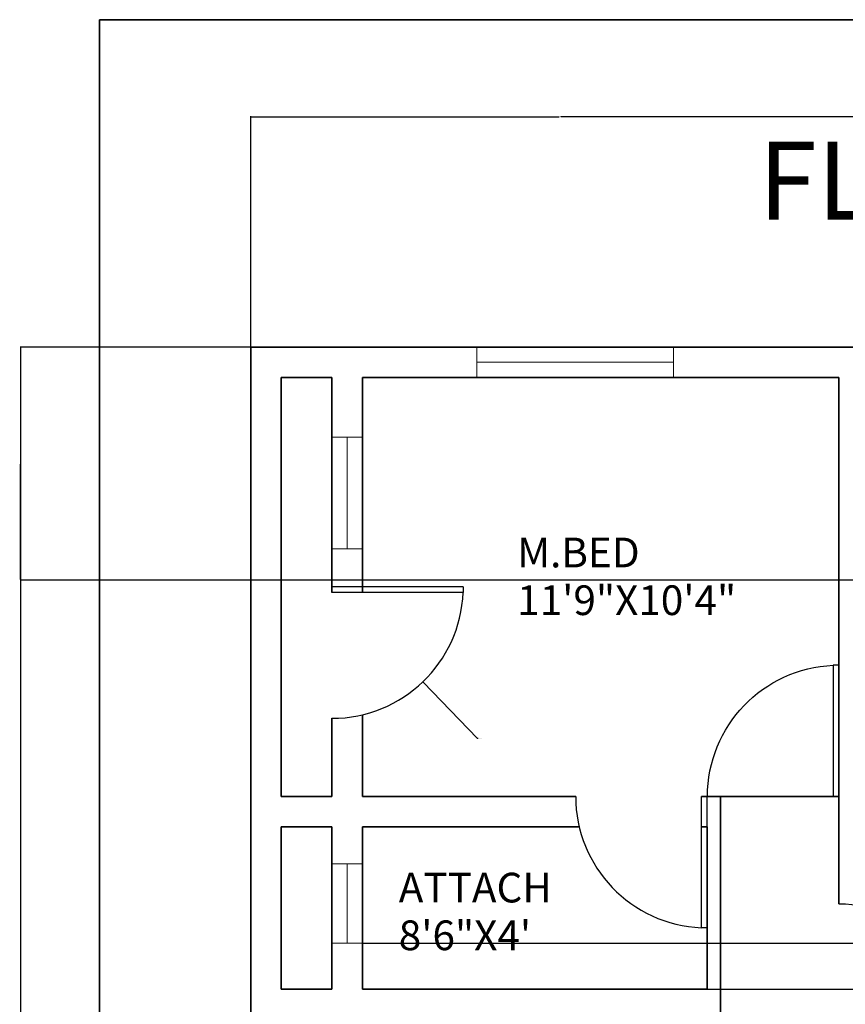
# Model space of a CAD drawing. Units: feet. Extents: x 100807 to 101423, y 154875 to 156331.
# Tile 3 of 8: x 100807 to 101051, y 156040 to 156331. Entities that reach past the tile are written whole.
import ezdxf

# ---------------------------------------------------------------- set-up
doc = ezdxf.new("R2010")
doc.units = ezdxf.units.FT
for name, color, linetype, lineweight in [('A-ANNO-DIMS', 2, 'Continuous', 18), ('A-ANNO-TITL', 7, 'Continuous', 35), ('A-ANNO-TTLB', 7, 'Continuous', 35), ('A-AREA-IDEN', 7, 'Continuous', 25), ('A-DOOR', 4, 'Continuous', 25), ('A-GLAZ', 4, 'Continuous', 18), ('A-WALL', 7, 'Continuous', 35)]:
    doc.layers.add(name, color=color, linetype=linetype, lineweight=lineweight)
doc.styles.get("Standard").update_dxf_attribs({"font": 'arial.ttf'})
doc.dimstyles.get("Standard").update_dxf_attribs({"dimtxt": 0.18, "dimasz": 0.18, "dimexe": 0.18, "dimexo": 0.0625, "dimgap": 0.09, "dimtad": 0, "dimtih": 1, "dimtoh": 1, "dimdec": 4, "dimzin": 0, "dimdsep": 46, "dimtxsty": 'Standard', "dimcen": 0.09, "dimadec": 0, "dimazin": 0, "dimtfac": 1, "dimtdec": 4, "dimtofl": 0, "dimtmove": 0, "dimatfit": 3, "dimfxl": 1, "dimtolj": 1, "dimtzin": 0, "dimarcsym": 0})

# ---------------------------------------------------------------- blocks, each defined once
blk = doc.blocks.new('DR-36')
for p, q in [((0, 36), (0, 0)), ((0, 36), (1.5, 36)), ((1.5, 36), (1.5, 0)), ((0, 0), (1.5, 0))]:
    blk.add_line(p, q)
blk.add_arc((0, 0), 36, 0, 87.6141)
blk = doc.blocks.new('WIN-BATH-SIDE')
for p, q in [((0, 23.54), (9, 23.54)), ((4.5, 23.54), (4.5, 0)), ((0, 0), (9, 0))]:
    blk.add_line(p, q)
blk = doc.blocks.new('WIN-MBED-SIDE')
for p, q in [((0, 33.08), (9, 33.08)), ((4.5, 33.08), (4.5, 0)), ((0, 0), (9, 0))]:
    blk.add_line(p, q)
blk = doc.blocks.new('*D35')
at = {"layer": 'A-ANNO-DIMS', "color": 0, "lineweight": -2, "transparency": 16777216}
for p, q in [((100875.09, 156234.58), (100806.83, 156234.58)), ((100807.01, 156234.4), (100807.01, 155589.76)), ((100807.01, 154944.76), (100807.01, 155589.4)), ((100875.09, 154944.58), (100806.83, 154944.58))]:
    blk.add_line(p, q, dxfattribs=at)
at = {"layer": 'A-ANNO-DIMS', "color": 0, "transparency": 16777216}
for points in [[(100806.98, 156234.4), (100807.04, 156234.4), (100807.01, 156234.58)], [(100806.98, 154944.76), (100807.04, 154944.76), (100807.01, 154944.58)]]:
    blk.add_solid(points, dxfattribs=at)
at = {"layer": 'Defpoints', "color": 0, "transparency": 16777216}
for p in [(100807.01, 156234.58), (100875.16, 156234.58), (100875.16, 154944.58)]:
    blk.add_point(p, dxfattribs=at)
at = {"layer": 'A-ANNO-DIMS', "color": 0, "transparency": 16777216, "insert": (100807.01, 155589.58), "char_height": 0.18, "attachment_point": 5}
blk.add_mtext('\\A1;1290', dxfattribs=at)
blk = doc.blocks.new('*D38')
at = {"layer": 'A-ANNO-DIMS', "color": 0, "lineweight": -2, "transparency": 16777216}
for p, q in [((100875.16, 156234.64), (100875.16, 156302.91)), ((100875.34, 156302.73), (100966.38, 156302.73)), ((101057.98, 156302.73), (100966.94, 156302.73)), ((101058.16, 156234.64), (101058.16, 156302.91))]:
    blk.add_line(p, q, dxfattribs=at)
at = {"layer": 'A-ANNO-DIMS', "color": 0, "transparency": 16777216}
for points in [[(100875.34, 156302.76), (100875.34, 156302.7), (100875.16, 156302.73)], [(101057.98, 156302.76), (101057.98, 156302.7), (101058.16, 156302.73)]]:
    blk.add_solid(points, dxfattribs=at)
at = {"layer": 'Defpoints', "color": 0, "transparency": 16777216}
for p in [(101058.16, 156302.73), (100875.16, 156234.58), (101058.16, 156234.58)]:
    blk.add_point(p, dxfattribs=at)
at = {"layer": 'A-ANNO-DIMS', "color": 0, "transparency": 16777216, "insert": (100966.66, 156302.73), "char_height": 0.18, "attachment_point": 5}
blk.add_mtext('\\A1;183', dxfattribs=at)
blk = doc.blocks.new('*D40')
at = {"layer": 'A-ANNO-DIMS', "color": 0, "lineweight": -2, "transparency": 16777216}
for p, q in [((101171.09, 156234.58), (100806.83, 156234.58)), ((100807.01, 156234.4), (100807.01, 156200.26)), ((100807.01, 156165.76), (100807.01, 156199.9)), ((101171.09, 156165.58), (100806.83, 156165.58))]:
    blk.add_line(p, q, dxfattribs=at)
at = {"layer": 'A-ANNO-DIMS', "color": 0, "transparency": 16777216}
for points in [[(100806.98, 156234.4), (100807.04, 156234.4), (100807.01, 156234.58)], [(100806.98, 156165.76), (100807.04, 156165.76), (100807.01, 156165.58)]]:
    blk.add_solid(points, dxfattribs=at)
at = {"layer": 'Defpoints', "color": 0, "transparency": 16777216}
for p in [(100807.01, 156234.58), (101171.16, 156234.58), (101171.16, 156165.58)]:
    blk.add_point(p, dxfattribs=at)
at = {"layer": 'A-ANNO-DIMS', "color": 0, "transparency": 16777216, "insert": (100807.01, 156200.08), "char_height": 0.18, "attachment_point": 5}
blk.add_mtext('\\A1;69', dxfattribs=at)
blk = doc.blocks.new('*D55')
at = {"layer": 'A-ANNO-DIMS', "color": 0, "lineweight": -2, "transparency": 16777216}
for p, q in [((100908.22, 156058.13), (101422.49, 156058.13)), ((101422.31, 156057.95), (101422.31, 156051.53)), ((101422.31, 156044.76), (101422.31, 156051.17)), ((100908.22, 156044.58), (101422.49, 156044.58))]:
    blk.add_line(p, q, dxfattribs=at)
at = {"layer": 'A-ANNO-DIMS', "color": 0, "transparency": 16777216}
for points in [[(101422.28, 156057.95), (101422.34, 156057.95), (101422.31, 156058.13)], [(101422.28, 156044.76), (101422.34, 156044.76), (101422.31, 156044.58)]]:
    blk.add_solid(points, dxfattribs=at)
at = {"layer": 'Defpoints', "color": 0, "transparency": 16777216}
for p in [(100908.16, 156058.13), (101422.31, 156058.13), (100908.16, 156044.58)]:
    blk.add_point(p, dxfattribs=at)
at = {"layer": 'A-ANNO-DIMS', "color": 0, "transparency": 16777216, "insert": (101422.31, 156051.35), "char_height": 0.18, "attachment_point": 5}
blk.add_mtext('\\A1;13.55', dxfattribs=at)
blk = doc.blocks.new('*D56')
at = {"layer": 'A-ANNO-DIMS', "color": 0, "lineweight": -2, "transparency": 16777216}
for p, q in [((100899.07, 156163.58), (100899.25, 156163.58)), ((100899.16, 156163.49), (100899.16, 156163.67)), ((100942.21, 156118.7), (100926.19, 156135.4)), ((100942.39, 156118.7), (100942.21, 156118.7))]:
    blk.add_line(p, q, dxfattribs=at)
at = {"layer": 'A-ANNO-DIMS', "color": 0, "transparency": 16777216}
blk.add_solid([(100926.21, 156135.42), (100926.17, 156135.38), (100926.06, 156135.53)], dxfattribs=at)
at = {"layer": 'Defpoints', "color": 0, "transparency": 16777216}
for p in [(100899.16, 156163.58), (100926.06, 156135.53)]:
    blk.add_point(p, dxfattribs=at)
at = {"layer": 'A-ANNO-DIMS', "color": 0, "transparency": 16777216, "insert": (100943.12, 156118.7), "char_height": 0.18, "attachment_point": 5}
blk.add_mtext('\\A1;15X R38.87', dxfattribs=at)

msp = doc.modelspace()

# ---------------------------------------------------------------- linework, layer by layer
at = {"layer": 'A-ANNO-TTLB'}
msp.add_lwpolyline([(100830.3877, 156331.4447), (101396.4426, 156331.4447), (101396.4426, 154875.4601), (100830.3877, 154875.4601)], close=True, dxfattribs=at)
at = {"layer": 'A-GLAZ'}
for p, q in [((100942.0128, 156234.5777), (100942.0128, 156225.5777)), ((101000.2489, 156234.5777), (101000.2489, 156225.5777)), ((100942.0128, 156230.0777), (101000.2489, 156230.0777))]:
    msp.add_line(p, q, dxfattribs=at)
at = {"layer": 'A-WALL'}
for p, q in [((100875.1564, 156234.5777), (101058.1564, 156234.5777)), ((100875.1564, 156035.5777), (100875.1564, 156234.5777)), ((100884.1564, 156225.5777), (100899.1564, 156225.5777)), ((100884.1564, 156101.5777), (100884.1564, 156225.5777)), ((100899.1564, 156161.9582), (100899.1564, 156225.5777)), ((100908.1564, 156225.5777), (101049.1564, 156225.5777)), ((100908.1564, 156161.9582), (100908.1564, 156225.5777)), ((101049.1564, 156225.5777), (101049.1564, 156101.5777)), ((100899.1564, 156101.5777), (100899.1564, 156124.7095)), ((100908.1564, 156101.5777), (100908.1564, 156125.7659)), ((100899.1564, 156101.5777), (100884.1564, 156101.5777)), ((100971.2882, 156101.5777), (100908.1564, 156101.5777)), ((101049.1564, 156101.5777), (101008.5369, 156101.5777)), ((101014.1564, 155945.4274), (101014.1564, 156101.5777)), ((101049.1564, 156101.5777), (101049.1564, 156069.8276)), ((100884.1564, 156044.5777), (100884.1564, 156092.5777)), ((100899.1564, 156092.5777), (100884.1564, 156092.5777)), ((100899.1564, 156092.5777), (100899.1564, 156044.5777)), ((100908.1564, 156092.5777), (100908.1564, 156044.5777)), ((100972.3446, 156092.5777), (100908.1564, 156092.5777)), ((101010.1564, 156092.5777), (101008.5369, 156092.5777)), ((101010.1564, 156044.5777), (101010.1564, 156092.5777)), ((101014.1564, 156044.5777), (101014.1564, 156092.5777)), ((100884.1564, 156044.5777), (100899.1564, 156044.5777)), ((100908.1564, 156044.5777), (101010.1564, 156044.5777))]:
    msp.add_line(p, q, dxfattribs=at)

# ---------------------------------------------------------------- block references
at = {"layer": 'A-DOOR', "yscale": 1.079672442471032, "zscale": 1.079672442471032}
for p, xscale, rotation in [((100899.1564, 156163.5777), 1.079672442471032, 269.9999999999631), ((101010.1564, 156101.5777), 1.079672442471032, 180), ((101049.1564, 156030.9594), -1.079672442471032, 270.0000000000369)]:
    msp.add_blockref('DR-36', p, dxfattribs=dict(at, xscale=xscale, rotation=rotation))
at = {"layer": 'A-DOOR', "xscale": -1.079672442471032, "yscale": 1.079672442471032, "zscale": 1.079672442471032}
msp.add_blockref('DR-36', (101049.1564, 156101.5777), dxfattribs=at)
at = {"layer": 'A-GLAZ'}
for name, p in [('WIN-MBED-SIDE', (100899.1564, 156174.8541)), ('WIN-BATH-SIDE', (100899.1564, 156058.1276))]:
    msp.add_blockref(name, p, dxfattribs=at)

# ---------------------------------------------------------------- texts
at = {"layer": 'A-ANNO-DIMS'}
for s, height, p in [('11\'9"X10\'4"', 8.788223, (100953.9752, 156155.2636)), ('8\'6"X4\'', 8.78822, (100918.9163, 156056.0978))]:
    msp.add_text(s, height=height, dxfattribs=at).set_placement(p)
at = {"layer": 'A-ANNO-TITL'}
msp.add_text('FLOOR PLAN', height=23.08638, dxfattribs=at).set_placement((101025.2804, 156272.2968))
at = {"layer": 'A-AREA-IDEN'}
for s, p in [('M.BED', (100953.9752, 156169.3811)), ('ATTACH', (100918.9163, 156070.2153))]:
    msp.add_text(s, height=8.78822, dxfattribs=at).set_placement(p)

# ---------------------------------------------------------------- dimensions: what is measured, and where the dimension line sits
at = {"layer": 'A-ANNO-DIMS'}
dim = msp.add_linear_dim(base=(101058.1564, 156302.7277), p1=(100875.1564, 156234.5777), p2=(101058.1564, 156234.5777), dimstyle='Standard', override={"dimdec": 0, "dimlfac": 1, "dimrnd": 0, "dimzin": 0, "dimdsep": 46, "dimlunit": 2}, dxfattribs=at)
dim.commit()
dim.dimension.update_dxf_attribs({"geometry": '*D38', "text_midpoint": (100966.6564, 156302.7277)})
for base, p1, p2, override, picture, middle in [((100807.0064, 156234.5777), (100875.1564, 154944.5777), (100875.1564, 156234.5777), {"dimdec": 0, "dimlfac": 1, "dimrnd": 0, "dimzin": 0, "dimdsep": 46, "dimlunit": 2}, '*D35', (100807.0064, 155589.5777)), ((100807.0064, 156234.5777), (101171.1564, 156165.5789), (101171.1564, 156234.5777), {"dimdec": 0, "dimlfac": 1, "dimrnd": 0, "dimzin": 0, "dimdsep": 46, "dimlunit": 2}, '*D40', (100807.0064, 156200.0783)), ((101422.3064, 156058.1276), (100908.1564, 156044.5777), (100908.1564, 156058.1276), {"dimdec": 2, "dimlfac": 1, "dimrnd": 0, "dimzin": 0, "dimdsep": 46, "dimlunit": 2}, '*D55', (101422.3064, 156051.3527))]:
    dim = msp.add_linear_dim(base=base, p1=p1, p2=p2, angle=90, dimstyle='Standard', override=override, dxfattribs=at)
    dim.commit()
    dim.dimension.update_dxf_attribs({"geometry": picture, "text_midpoint": middle})
dim = msp.add_radius_dim(center=(100899.1564, 156163.5777), mpoint=(100926.0624, 156135.5276), text='15X <>', dimstyle='Standard', override={"dimdec": 2, "dimlfac": 1, "dimrnd": 0, "dimzin": 0, "dimdsep": 46, "dimlunit": 2}, dxfattribs=at)
dim.commit()
dim.dimension.update_dxf_attribs({"geometry": '*D56', "text_midpoint": (100943.1206, 156118.6976), "dimtype": 164})

doc.saveas('drawing.dxf')
